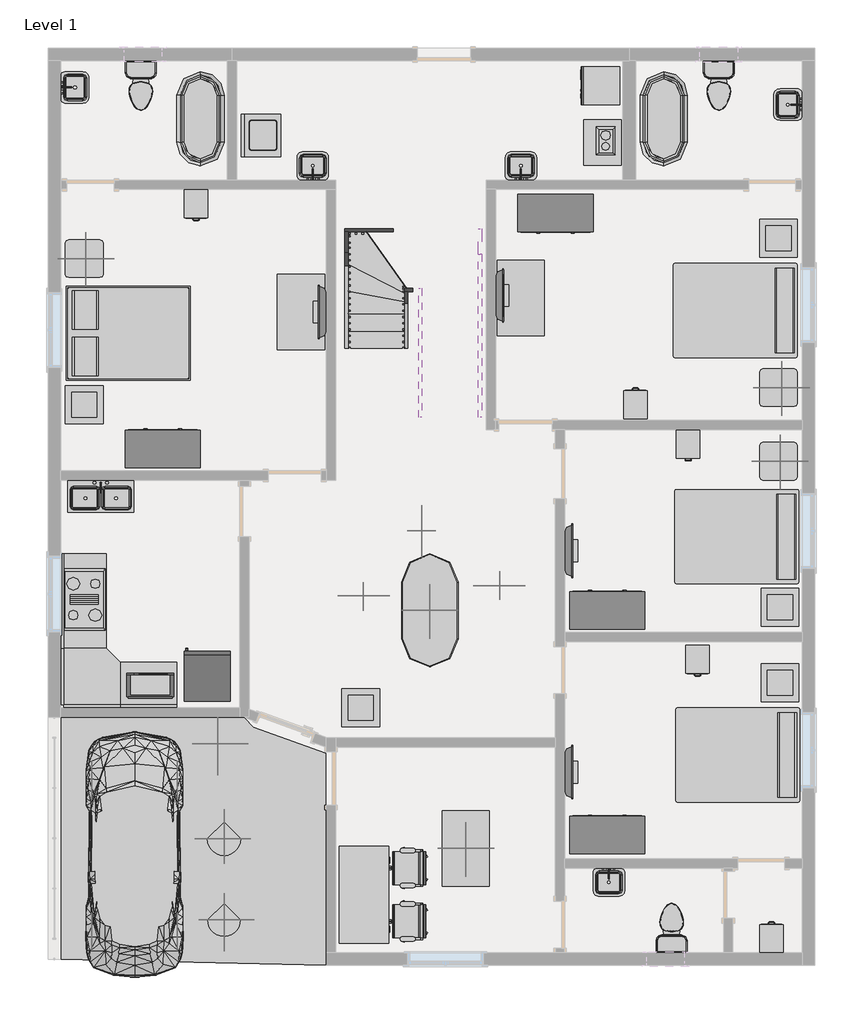
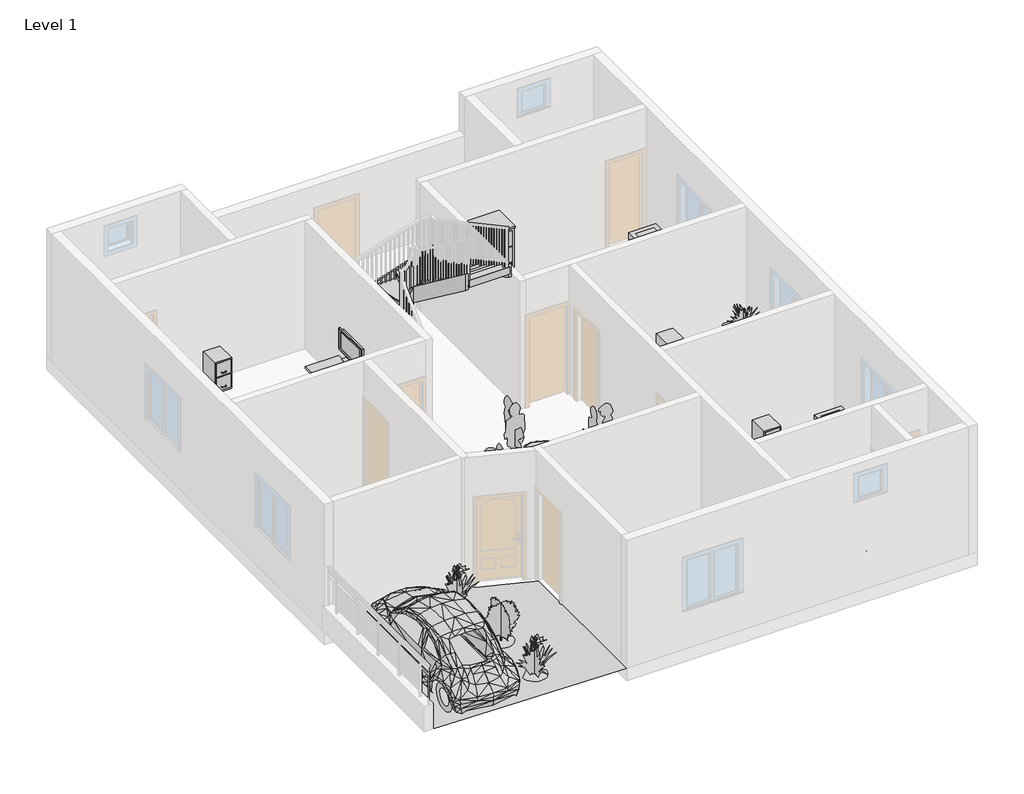
# One storey, part 3 of 3: 34 furniture elements, 15 flow terminals, 11 proxies, 8 geographic elements, 8 members, 1 stair flight.
"""IFC4 building model written with IfcOpenShell, lengths in millimetres."""

from ifc_helpers import new_model, si_unit, frame, origin, place, context, project, spatial, polyline, outline, extrude, triangles, transform, mapped, element, save
from components import proxy_fe84b772, proxy_bb1e6e30, proxy_45b28599, proxy_8a8d5ab2, rpc_beetle_rpc_beetle_3ce7ba48, rpc_female_69e001fa, proxy_a13a33b2, proxy_718fa39f, flow_terminal_2b63360b, flow_terminal_accce45a, flow_terminal_a53be723, flow_terminal_62a433f7, toilet_domestic_3d_toilet_domestic_3d_f7549cf7, toilet_domestic_3d_toilet_domestic_3d_183bbd19, flow_terminal_b374fae2, furniture_1d2926bd, furniture_e1791683, furniture_bb55ed6b, furniture_552c1472, chair_task_arms_chair_task_arms_fa5a08ef, furniture_072f6425, furniture_9fa109b2, furniture_56245f3a, furniture_b5c51a22, furniture_2c34a4f9, furniture_31d08a24, furniture_d260d85f, furniture_6a32cbcf, furniture_9653231d, rpc_plant_tropical_55f6ff97, rpc_plant_tropical_agave_1_5_93a2a214, rpc_plant_tropical_jungle_flame_3_9c4808c2, stair_flight_4b05d3ae

model = new_model("IFC4")

# Units and contexts
model_context = context("Model", 3, world=origin())
ifc_project = project(units=[si_unit("LENGTHUNIT", "METRE", prefix="MILLI")], contexts=[model_context])

# Site, building, storey
site = spatial("IfcSite", under=ifc_project)
building = spatial("IfcBuilding", under=site)
storey = spatial("IfcBuildingStorey", under=building, Name="Level 1", Elevation=0.0)

# Proxies
placement = place(None, origin())
element("IfcBuildingElementProxy", 1, Name="Building Element Proxy", at=placement, inside=storey, context=model_context, shape_type="Tessellation", body=[
    triangles([(-14773.0750122, 3106.6452576, 0.0), (-11814.7102386, 3106.6452576, 0.0), (-10480.4742371, 2547.8453545, 0.0), (-10480.4742371, 1684.245306, 0.0), (-10480.4742371, -906.5547667, 0.0), (-14773.0750122, -804.9547909, 0.0), (-10378.8746246, 1684.245306, 0.0), (-10378.8746246, 2547.8453545, 0.0), (-11521.9792694, 3081.190416, 0.0)], [[2, 4, 9], [4, 2, 6], [2, 1, 6], [4, 5, 7], [5, 4, 6], [3, 7, 8], [7, 3, 4], [3, 8, 9], [4, 3, 9]], closed=False),
])
proxy_shape = proxy_fe84b772(model_context)
element("IfcBuildingElementProxy", 2, Name="Cook Top-2 Unit : 12\" x 18\"", ObjectType="Cook Top-2 Unit : 12\" x 18\"", at=placement, inside=storey, context=model_context, shape_type="MappedRepresentation", body=[
    mapped(proxy_shape, transform((-6035.4744419, 12398.2204454, 0.0), x_axis=(1.0000000000000007, 0.0, 0.0), y_axis=(0.0, 1.0000000000000007, 0.0), z_axis=(0.0, 0.0, 1.0))),
])
proxy_2_shape = proxy_bb1e6e30(model_context)
element("IfcBuildingElementProxy", 3, Name="Cook Top-4 Unit : 36\" x 20\"", ObjectType="Cook Top-4 Unit : 36\" x 20\"", at=placement, inside=storey, context=model_context, shape_type="MappedRepresentation", body=[
    mapped(proxy_2_shape, transform((-14392.0744419, 5011.6452409, 0.0), x_axis=(0.0, 1.0, 0.0), y_axis=(-1.0, 0.0, 0.0), z_axis=(0.0, 0.0, 1.0))),
])
proxy_3_shape = proxy_45b28599(model_context)
element("IfcBuildingElementProxy", 4, Name="Dishwasher : 24\" x 24\" x 34\"", ObjectType="Dishwasher : 24\" x 24\" x 34\"", at=placement, inside=storey, context=model_context, shape_type="MappedRepresentation", body=[
    mapped(proxy_3_shape, transform((-6301.9240067, 13699.7627094, 0.0), x_axis=(0.0, -1.0000000000000004, 0.0), y_axis=(1.0000000000000004, 0.0, 0.0), z_axis=(0.0, 0.0, 1.0))),
])
proxy_4_shape = proxy_8a8d5ab2(model_context)
element("IfcBuildingElementProxy", 5, Name="Microwave : 30\" x 16\" x 18\"", ObjectType="Microwave : 30\" x 16\" x 18\"", at=placement, inside=storey, context=model_context, shape_type="MappedRepresentation", body=[
    mapped(proxy_4_shape, transform((-12824.9815646, 3261.5647351, 0.0), x_axis=(-1.0000000000000004, 0.0, 0.0), y_axis=(0.0, -1.0000000000000004, 0.0), z_axis=(0.0, 0.0, 1.0))),
])
rpc_beetle_rpc_beetle_shape = rpc_beetle_rpc_beetle_3ce7ba48(model_context)
element("IfcBuildingElementProxy", 6, Name="RPC Beetle : RPC Beetle", ObjectType="RPC Beetle : RPC Beetle", at=placement, inside=storey, context=model_context, shape_type="MappedRepresentation", body=[
    mapped(rpc_beetle_rpc_beetle_shape, transform((-13579.2744419, -347.7547591, 0.0), x_axis=(1.0, 0.0, 0.0), y_axis=(0.0, 1.0, 0.0), z_axis=(0.0, 0.0, 1.0))),
])
rpc_female_shape = rpc_female_69e001fa(model_context)
element("IfcBuildingElementProxy", 7, Name="RPC Female", ObjectType="RPC Female", at=placement, inside=storey, context=model_context, shape_type="MappedRepresentation", body=[
    mapped(rpc_female_shape, transform((-9721.6494419, 5062.4452409, 0.0), x_axis=(0.0, 1.0000000000000002, 0.0), y_axis=(-1.0000000000000002, 0.0, 0.0), z_axis=(0.0, 0.0, 1.0))),
])
element("IfcBuildingElementProxy", 8, Name="RPC Female", ObjectType="RPC Female", at=placement, inside=storey, context=model_context, shape_type="MappedRepresentation", body=[
    mapped(rpc_female_shape, transform((-8940.5994419, 5964.1452409, 0.0), x_axis=(1.0, 0.0, 0.0), y_axis=(0.0, 1.0, 0.0), z_axis=(0.0, 0.0, 1.0))),
])
element("IfcBuildingElementProxy", 9, Name="RPC Female", ObjectType="RPC Female", at=placement, inside=storey, context=model_context, shape_type="MappedRepresentation", body=[
    mapped(rpc_female_shape, transform((-7829.3494419, 5240.2452409, 0.0), x_axis=(0.0, -1.0000000000000007, 0.0), y_axis=(1.0000000000000007, 0.0, 0.0), z_axis=(0.0, 0.0, 1.0))),
])
proxy_5_shape = proxy_a13a33b2(model_context)
element("IfcBuildingElementProxy", 10, Name="Refrigerator : 30\" x 32\" RH", ObjectType="Refrigerator : 30\" x 32\" RH", at=placement, inside=storey, context=model_context, shape_type="MappedRepresentation", body=[
    mapped(proxy_5_shape, transform((-12402.9369419, 3753.1462695, 0.0), x_axis=(-1.0000000000000004, 0.0, 0.0), y_axis=(0.0, -1.0000000000000004, 0.0), z_axis=(0.0, 0.0, 1.0))),
])
proxy_6_shape = proxy_718fa39f(model_context)
element("IfcBuildingElementProxy", 11, Name="Washer : 27\" x 25\" x 35\"", ObjectType="Washer : 27\" x 25\" x 35\"", at=placement, inside=storey, context=model_context, shape_type="MappedRepresentation", body=[
    mapped(proxy_6_shape, transform((-11255.4248771, 12096.9277724, 0.0), x_axis=(0.0, 1.0000000000000004, 0.0), y_axis=(-1.0000000000000004, 0.0, 0.0), z_axis=(0.0, 0.0, 1.0))),
])

# Flow terminals
flow_terminal_shape = flow_terminal_2b63360b(model_context)
element("IfcFlowTerminal", 12, ObjectType="Floor Drain - Rectangular : 5\"x5\" Strainer - 2\" Drain", at=placement, inside=storey, context=model_context, shape_type="MappedRepresentation", body=[
    mapped(flow_terminal_shape, transform((-13122.0744419, 12022.0452409, 0.0), x_axis=(1.0, 0.0, 0.0), y_axis=(0.0, 1.0, 0.0), z_axis=(0.0, 0.0, 1.0))),
])
element("IfcFlowTerminal", 13, ObjectType="Floor Drain - Rectangular : 5\"x5\" Strainer - 2\" Drain", at=placement, inside=storey, context=model_context, shape_type="MappedRepresentation", body=[
    mapped(flow_terminal_shape, transform((-11598.0744419, 13368.2452409, 0.0), x_axis=(1.0, 0.0, 0.0), y_axis=(0.0, 1.0, 0.0), z_axis=(0.0, 0.0, 1.0))),
])
element("IfcFlowTerminal", 14, ObjectType="Floor Drain - Rectangular : 5\"x5\" Strainer - 2\" Drain", at=placement, inside=storey, context=model_context, shape_type="MappedRepresentation", body=[
    mapped(flow_terminal_shape, transform((-4460.6744419, 12225.2452409, 0.0), x_axis=(1.0, 0.0, 0.0), y_axis=(0.0, 1.0, 0.0), z_axis=(0.0, 0.0, 1.0))),
])
flow_terminal_2_shape = flow_terminal_accce45a(model_context)
element("IfcFlowTerminal", 15, ObjectType="Floor Drain - Round : 5\" Strainer - 2\" Drain", at=placement, inside=storey, context=model_context, shape_type="MappedRepresentation", body=[
    mapped(flow_terminal_2_shape, transform((-5425.8744419, -208.6587317, 0.0), x_axis=(1.0, 0.0, 0.0), y_axis=(0.0, 1.0, 0.0), z_axis=(0.0, 0.0, 1.0))),
])
flow_terminal_3_shape = flow_terminal_a53be723(model_context)
element("IfcFlowTerminal", 16, ObjectType="Sink Kitchen-Double : 42\" x 21\"", at=placement, inside=storey, context=model_context, shape_type="MappedRepresentation", body=[
    mapped(flow_terminal_3_shape, transform((-14141.0636825, 6685.6998398, 0.0), x_axis=(1.0, 0.0, 0.0), y_axis=(0.0, 1.0, 0.0), z_axis=(0.0, 0.0, 1.0))),
])
flow_terminal_4_shape = flow_terminal_62a433f7(model_context)
element("IfcFlowTerminal", 17, ObjectType="Sink Vanity-Square : 20\" x 18\"", at=placement, inside=storey, context=model_context, shape_type="MappedRepresentation", body=[
    mapped(flow_terminal_4_shape, transform((-14592.9290408, 13276.3560004, 0.0), x_axis=(0.0, 1.0000000000000002, 0.0), y_axis=(-1.0000000000000002, 0.0, 0.0), z_axis=(0.0, 0.0, 1.0))),
])
element("IfcFlowTerminal", 18, ObjectType="Sink Vanity-Square : 20\" x 18\"", at=placement, inside=storey, context=model_context, shape_type="MappedRepresentation", body=[
    mapped(flow_terminal_4_shape, transform((-10680.6852013, 11973.5906421, 0.0), x_axis=(-1.0, 0.0, 0.0), y_axis=(0.0, -1.0, 0.0), z_axis=(0.0, 0.0, 1.0))),
])
element("IfcFlowTerminal", 19, ObjectType="Sink Vanity-Square : 20\" x 18\"", at=placement, inside=storey, context=model_context, shape_type="MappedRepresentation", body=[
    mapped(flow_terminal_4_shape, transform((-7315.1852013, 11973.5906421, 0.0), x_axis=(-0.9999999999999998, 0.0, 0.0), y_axis=(0.0, -0.9999999999999998, 0.0), z_axis=(0.0, 0.0, 1.0))),
])
element("IfcFlowTerminal", 20, ObjectType="Sink Vanity-Square : 20\" x 18\"", at=placement, inside=storey, context=model_context, shape_type="MappedRepresentation", body=[
    mapped(flow_terminal_4_shape, transform((-2964.419843, 13028.3344815, 0.0), x_axis=(0.0, -1.0000000000000004, 0.0), y_axis=(1.0000000000000004, 0.0, 0.0), z_axis=(0.0, 0.0, 1.0))),
])
element("IfcFlowTerminal", 21, ObjectType="Sink Vanity-Square : 20\" x 18\"", at=placement, inside=storey, context=model_context, shape_type="MappedRepresentation", body=[
    mapped(flow_terminal_4_shape, transform((-5924.1636825, 488.0998398, 0.0), x_axis=(1.0, 0.0, 0.0), y_axis=(0.0, 1.0, 0.0), z_axis=(0.0, 0.0, 1.0))),
])
toilet_domestic_3d_toilet_domestic_3d_shape = toilet_domestic_3d_toilet_domestic_3d_f7549cf7(model_context)
toilet_domestic_3d_toilet_domestic_3d_2_shape = toilet_domestic_3d_toilet_domestic_3d_183bbd19(model_context)
element("IfcFlowTerminal", 22, ObjectType="Toilet-Domestic-3D : Toilet-Domestic-3D", at=placement, inside=storey, context=model_context, shape_type="MappedRepresentation", body=[
    mapped(toilet_domestic_3d_toilet_domestic_3d_shape, transform((-13477.6744419, 13229.1492136, 0.0), x_axis=(1.0, 0.0, 0.0), y_axis=(0.0, 1.0, 0.0), z_axis=(0.0, 0.0, 1.0))),
    mapped(toilet_domestic_3d_toilet_domestic_3d_2_shape, transform((-13477.6744419, 13229.1492136, 0.0), x_axis=(1.0, 0.0, 0.0), y_axis=(0.0, 1.0, 0.0), z_axis=(0.0, 0.0, 1.0))),
])
element("IfcFlowTerminal", 23, ObjectType="Toilet-Domestic-3D : Toilet-Domestic-3D", at=placement, inside=storey, context=model_context, shape_type="MappedRepresentation", body=[
    mapped(toilet_domestic_3d_toilet_domestic_3d_shape, transform((-4130.4744419, 13229.1492136, 0.0), x_axis=(1.0, 0.0, 0.0), y_axis=(0.0, 1.0, 0.0), z_axis=(0.0, 0.0, 1.0))),
    mapped(toilet_domestic_3d_toilet_domestic_3d_2_shape, transform((-4130.4744419, 13229.1492136, 0.0), x_axis=(1.0, 0.0, 0.0), y_axis=(0.0, 1.0, 0.0), z_axis=(0.0, 0.0, 1.0))),
])
element("IfcFlowTerminal", 24, ObjectType="Toilet-Domestic-3D : Toilet-Domestic-3D", at=placement, inside=storey, context=model_context, shape_type="MappedRepresentation", body=[
    mapped(toilet_domestic_3d_toilet_domestic_3d_shape, transform((-4892.4744419, -208.6587317, 0.0), x_axis=(-1.0000000000000004, 0.0, 0.0), y_axis=(0.0, -1.0000000000000004, 0.0), z_axis=(0.0, 0.0, 1.0))),
    mapped(toilet_domestic_3d_toilet_domestic_3d_2_shape, transform((-4892.4744419, -208.6587317, 0.0), x_axis=(-1.0000000000000004, 0.0, 0.0), y_axis=(0.0, -1.0000000000000004, 0.0), z_axis=(0.0, 0.0, 1.0))),
])
flow_terminal_5_shape = flow_terminal_b374fae2(model_context)
element("IfcFlowTerminal", 25, ObjectType="Tub-Free Standing-3D : 30\" x 60\"", at=placement, inside=storey, context=model_context, shape_type="MappedRepresentation", body=[
    mapped(flow_terminal_5_shape, transform((-12512.4744419, 12784.0452409, 0.0), x_axis=(1.0, 0.0, 0.0), y_axis=(0.0, 1.0, 0.0), z_axis=(0.0, 0.0, 1.0))),
])
element("IfcFlowTerminal", 26, ObjectType="Tub-Free Standing-3D : 30\" x 60\"", at=placement, inside=storey, context=model_context, shape_type="MappedRepresentation", body=[
    mapped(flow_terminal_5_shape, transform((-5019.4744419, 12784.0452409, 0.0), x_axis=(1.0, 0.0, 0.0), y_axis=(0.0, 1.0, 0.0), z_axis=(0.0, 0.0, 1.0))),
])

# Furniture
furniture_shape = furniture_1d2926bd(model_context)
element("IfcFurniture", 27, ObjectType="Bed-Box : Queen 60\" x 79\"", at=placement, inside=storey, context=model_context, shape_type="MappedRepresentation", body=[
    mapped(furniture_shape, transform((-13915.3039501, 8977.7927819, 0.0), x_axis=(0.0, 1.0000000000000002, 0.0), y_axis=(-1.0000000000000002, 0.0, 0.0), z_axis=(0.0, 0.0, 1.0))),
])
furniture_2_shape = furniture_e1791683(model_context)
element("IfcFurniture", 28, ObjectType="Bed-Standard.0001 : Queen 60\" x 79\"", at=placement, inside=storey, context=model_context, shape_type="MappedRepresentation", body=[
    mapped(furniture_2_shape, transform((-3818.1793599, 9956.7337655, 0.0), x_axis=(0.0, -1.0, 0.0), y_axis=(1.0, 0.0, 0.0), z_axis=(0.0, 0.0, 1.0))),
])
element("IfcFurniture", 29, ObjectType="Bed-Standard.0001 : Queen 60\" x 79\"", at=placement, inside=storey, context=model_context, shape_type="MappedRepresentation", body=[
    mapped(furniture_2_shape, transform((-3792.7793599, 6299.1337655, 0.0), x_axis=(0.0, -1.0000000000000002, 0.0), y_axis=(1.0000000000000002, 0.0, 0.0), z_axis=(0.0, 0.0, 1.0))),
])
element("IfcFurniture", 30, ObjectType="Bed-Standard.0001 : Queen 60\" x 79\"", at=placement, inside=storey, context=model_context, shape_type="MappedRepresentation", body=[
    mapped(furniture_2_shape, transform((-3780.0793599, 2768.5337655, 0.0), x_axis=(0.0, -1.0, 0.0), y_axis=(1.0, 0.0, 0.0), z_axis=(0.0, 0.0, 1.0))),
])
furniture_3_shape = furniture_bb55ed6b(model_context)
element("IfcFurniture", 31, ObjectType="Cabinet-File 2 Drawer : 15\" x 18\"", at=placement, inside=storey, context=model_context, shape_type="MappedRepresentation", body=[
    mapped(furniture_3_shape, transform((-12454.7220198, 11554.5795411, 0.0), x_axis=(1.0, 0.0, 0.0), y_axis=(0.0, 1.0, 0.0), z_axis=(0.0, 0.0, 1.0))),
])
element("IfcFurniture", 32, ObjectType="Cabinet-File 2 Drawer : 15\" x 18\"", at=placement, inside=storey, context=model_context, shape_type="MappedRepresentation", body=[
    mapped(furniture_3_shape, transform((-5604.5708889, 8019.1109408, 0.0), x_axis=(-1.0, 0.0, 0.0), y_axis=(0.0, -1.0, 0.0), z_axis=(0.0, 0.0, 1.0))),
])
element("IfcFurniture", 33, ObjectType="Cabinet-File 2 Drawer : 15\" x 18\"", at=placement, inside=storey, context=model_context, shape_type="MappedRepresentation", body=[
    mapped(furniture_3_shape, transform((-4497.8779949, 7668.3795411, 0.0), x_axis=(1.0, 0.0, 0.0), y_axis=(0.0, 1.0, 0.0), z_axis=(0.0, 0.0, 1.0))),
])
element("IfcFurniture", 34, ObjectType="Cabinet-File 2 Drawer : 15\" x 18\"", at=placement, inside=storey, context=model_context, shape_type="MappedRepresentation", body=[
    mapped(furniture_3_shape, transform((-4345.4779949, 4188.5795411, 0.0), x_axis=(1.0, 0.0, 0.0), y_axis=(0.0, 1.0, 0.0), z_axis=(0.0, 0.0, 1.0))),
])
furniture_4_shape = furniture_552c1472(model_context)
element("IfcFurniture", 35, ObjectType="Cabinet-File 3 Drawer : 15\" x 18\"", at=placement, inside=storey, context=model_context, shape_type="MappedRepresentation", body=[
    mapped(furniture_4_shape, transform((-3407.4708889, -616.8890592, 0.0), x_axis=(-1.0000000000000004, 0.0, 0.0), y_axis=(0.0, -1.0000000000000004, 0.0), z_axis=(0.0, 0.0, 1.0))),
])
chair_task_arms_chair_task_arms_shape = chair_task_arms_chair_task_arms_fa5a08ef(model_context)
element("IfcFurniture", 36, ObjectType="Chair-Task Arms : Chair-Task Arms", at=placement, inside=storey, context=model_context, shape_type="MappedRepresentation", body=[
    mapped(chair_task_arms_chair_task_arms_shape, transform((-9115.3285403, -336.3455787, 0.0), x_axis=(0.0, 1.0, 0.0), y_axis=(-1.0, 0.0, 0.0), z_axis=(0.0, 0.0, 1.0))),
])
element("IfcFurniture", 37, ObjectType="Chair-Task Arms : Chair-Task Arms", at=placement, inside=storey, context=model_context, shape_type="MappedRepresentation", body=[
    mapped(chair_task_arms_chair_task_arms_shape, transform((-9115.3285403, 527.2544213, 0.0), x_axis=(0.0, 1.0000000000000002, 0.0), y_axis=(-1.0000000000000002, 0.0, 0.0), z_axis=(0.0, 0.0, 1.0))),
])
furniture_5_shape = furniture_072f6425(model_context)
element("IfcFurniture", 38, ObjectType="Desk : 60\" x 30\" Student", at=placement, inside=storey, context=model_context, shape_type="MappedRepresentation", body=[
    mapped(furniture_5_shape, transform((-10251.8744419, 998.4452409, 0.0), x_axis=(0.0, -1.0000000000000007, 0.0), y_axis=(1.0000000000000007, 0.0, 0.0), z_axis=(0.0, 0.0, 1.0))),
])
furniture_6_shape = furniture_9fa109b2(model_context)
element("IfcFurniture", 39, ObjectType="Dresser : 48\" x 72\" x 24\"", at=placement, inside=storey, context=model_context, shape_type="MappedRepresentation", body=[
    mapped(furniture_6_shape, transform((-13391.2677017, 7083.150595, 0.0), x_axis=(-1.0000000000000004, 0.0, 0.0), y_axis=(0.0, -1.0000000000000004, 0.0), z_axis=(0.0, 0.0, 1.0))),
])
element("IfcFurniture", 40, ObjectType="Dresser : 48\" x 72\" x 24\"", at=placement, inside=storey, context=model_context, shape_type="MappedRepresentation", body=[
    mapped(furniture_6_shape, transform((-6502.8811821, 11623.208195, 0.0), x_axis=(1.0, 0.0, 0.0), y_axis=(0.0, 1.0, 0.0), z_axis=(0.0, 0.0, 1.0))),
])
element("IfcFurniture", 41, ObjectType="Dresser : 48\" x 72\" x 24\"", at=placement, inside=storey, context=model_context, shape_type="MappedRepresentation", body=[
    mapped(furniture_6_shape, transform((-6203.0677017, 4470.6822868, 0.0), x_axis=(-1.0000000000000004, 0.0, 0.0), y_axis=(0.0, -1.0000000000000004, 0.0), z_axis=(0.0, 0.0, 1.0))),
])
element("IfcFurniture", 42, ObjectType="Dresser : 48\" x 72\" x 24\"", at=placement, inside=storey, context=model_context, shape_type="MappedRepresentation", body=[
    mapped(furniture_6_shape, transform((-6203.0677017, 838.4822868, 0.0), x_axis=(-1.0000000000000004, 0.0, 0.0), y_axis=(0.0, -1.0000000000000004, 0.0), z_axis=(0.0, 0.0, 1.0))),
])
furniture_7_shape = furniture_56245f3a(model_context)
element("IfcFurniture", 43, ObjectType="TV - Flat Screen : 32\"", at=placement, inside=storey, context=model_context, shape_type="MappedRepresentation", body=[
    mapped(furniture_7_shape, transform((-10539.0130656, 9655.9007268, 914.4), x_axis=(0.0, -1.0000000000000004, 0.0), y_axis=(1.0000000000000004, 0.0, 0.0), z_axis=(0.0, 0.0, 1.0))),
])
element("IfcFurniture", 44, ObjectType="TV - Flat Screen : 32\"", at=placement, inside=storey, context=model_context, shape_type="MappedRepresentation", body=[
    mapped(furniture_7_shape, transform((-7678.7358183, 9930.4897551, 990.6), x_axis=(0.0, 1.0000000000000002, 0.0), y_axis=(-1.0000000000000002, 0.0, 0.0), z_axis=(0.0, 0.0, 1.0))),
])
element("IfcFurniture", 45, ObjectType="TV - Flat Screen : 32\"", at=placement, inside=storey, context=model_context, shape_type="MappedRepresentation", body=[
    mapped(furniture_7_shape, transform((-6561.1358183, 5802.9897551, 914.4), x_axis=(0.0, 1.0, 0.0), y_axis=(-1.0, 0.0, 0.0), z_axis=(0.0, 0.0, 1.0))),
])
element("IfcFurniture", 46, ObjectType="TV - Flat Screen : 32\"", at=placement, inside=storey, context=model_context, shape_type="MappedRepresentation", body=[
    mapped(furniture_7_shape, transform((-6561.1358183, 2221.5897551, 914.4), x_axis=(0.0, 1.0, 0.0), y_axis=(-1.0, 0.0, 0.0), z_axis=(0.0, 0.0, 1.0))),
])
furniture_8_shape = furniture_b5c51a22(model_context)
element("IfcFurniture", 47, ObjectType="Table-Coffee : 24\" x 24\" x 24\"", at=placement, inside=storey, context=model_context, shape_type="MappedRepresentation", body=[
    mapped(furniture_8_shape, transform((-14410.3402086, 8066.0341631, 0.0), x_axis=(1.0, 0.0, 0.0), y_axis=(0.0, 1.0, 0.0), z_axis=(0.0, 0.0, 1.0))),
])
element("IfcFurniture", 48, ObjectType="Table-Coffee : 24\" x 24\" x 24\"", at=placement, inside=storey, context=model_context, shape_type="MappedRepresentation", body=[
    mapped(furniture_8_shape, transform((-3183.5402086, 10758.4341631, 0.0), x_axis=(1.0, 0.0, 0.0), y_axis=(0.0, 1.0, 0.0), z_axis=(0.0, 0.0, 1.0))),
])
element("IfcFurniture", 49, ObjectType="Table-Coffee : 24\" x 24\" x 24\"", at=placement, inside=storey, context=model_context, shape_type="MappedRepresentation", body=[
    mapped(furniture_8_shape, transform((-9939.9402086, 3163.8341631, 0.0), x_axis=(1.0, 0.0, 0.0), y_axis=(0.0, 1.0, 0.0), z_axis=(0.0, 0.0, 1.0))),
])
element("IfcFurniture", 50, ObjectType="Table-Coffee : 24\" x 24\" x 24\"", at=placement, inside=storey, context=model_context, shape_type="MappedRepresentation", body=[
    mapped(furniture_8_shape, transform((-3158.1402086, 4789.4341631, 0.0), x_axis=(1.0, 0.0, 0.0), y_axis=(0.0, 1.0, 0.0), z_axis=(0.0, 0.0, 1.0))),
])
element("IfcFurniture", 51, ObjectType="Table-Coffee : 24\" x 24\" x 24\"", at=placement, inside=storey, context=model_context, shape_type="MappedRepresentation", body=[
    mapped(furniture_8_shape, transform((-3158.1402086, 3570.2341631, 0.0), x_axis=(1.0, 0.0, 0.0), y_axis=(0.0, 1.0, 0.0), z_axis=(0.0, 0.0, 1.0))),
])
furniture_9_shape = furniture_2c34a4f9(model_context)
element("IfcFurniture", 52, ObjectType="Table-Dining Oval : 36\" x 72\"", at=placement, inside=storey, context=model_context, shape_type="MappedRepresentation", body=[
    mapped(furniture_9_shape, transform((-9162.1728026, 5235.6649131, 0.0), x_axis=(0.0, 1.0, 0.0), y_axis=(-1.0, 0.0, 0.0), z_axis=(0.0, 0.0, 1.0))),
])
furniture_10_shape = furniture_31d08a24(model_context)
element("IfcFurniture", 53, ObjectType="Table-End : 24\" x 24\"", at=placement, inside=storey, context=model_context, shape_type="MappedRepresentation", body=[
    mapped(furniture_10_shape, transform((-14700.6080722, 10371.0452409, 0.0), x_axis=(1.0, 0.0, 0.0), y_axis=(0.0, 1.0, 0.0), z_axis=(0.0, 0.0, 1.0))),
])
element("IfcFurniture", 54, ObjectType="Table-End : 24\" x 24\"", at=placement, inside=storey, context=model_context, shape_type="MappedRepresentation", body=[
    mapped(furniture_10_shape, transform((-3473.8080722, 8284.5135491, 0.0), x_axis=(1.0, 0.0, 0.0), y_axis=(0.0, 1.0, 0.0), z_axis=(0.0, 0.0, 1.0))),
])
element("IfcFurniture", 55, ObjectType="Table-End : 24\" x 24\"", at=placement, inside=storey, context=model_context, shape_type="MappedRepresentation", body=[
    mapped(furniture_10_shape, transform((-3473.8080722, 7094.4452409, 0.0), x_axis=(1.0, 0.0, 0.0), y_axis=(0.0, 1.0, 0.0), z_axis=(0.0, 0.0, 1.0))),
])
furniture_11_shape = furniture_d260d85f(model_context)
element("IfcFurniture", 56, ObjectType="Table-Rectangular : 72\" x 30\" 2", at=placement, inside=storey, context=model_context, shape_type="MappedRepresentation", body=[
    mapped(furniture_11_shape, transform((-10886.8744419, 9659.8452409, 0.0), x_axis=(0.0, 1.0000000000000002, 0.0), y_axis=(-1.0000000000000002, 0.0, 0.0), z_axis=(0.0, 0.0, 1.0))),
])
element("IfcFurniture", 57, ObjectType="Table-Rectangular : 72\" x 30\" 2", at=placement, inside=storey, context=model_context, shape_type="MappedRepresentation", body=[
    mapped(furniture_11_shape, transform((-7330.8744419, 9888.4452409, 0.0), x_axis=(0.0, 1.0000000000000002, 0.0), y_axis=(-1.0000000000000002, 0.0, 0.0), z_axis=(0.0, 0.0, 1.0))),
])
element("IfcFurniture", 58, ObjectType="Table-Rectangular : 72\" x 30\" 2", at=placement, inside=storey, context=model_context, shape_type="MappedRepresentation", body=[
    mapped(furniture_11_shape, transform((-8219.8744419, 985.7452409, 0.0), x_axis=(0.0, 1.0, 0.0), y_axis=(-1.0, 0.0, 0.0), z_axis=(0.0, 0.0, 1.0))),
])
furniture_12_shape = furniture_6a32cbcf(model_context)
element("IfcFurniture", 59, ObjectType="Table-Rectangular : 72\" x 30\" 3", at=placement, inside=storey, context=model_context, shape_type="MappedRepresentation", body=[
    mapped(furniture_12_shape, transform((-6010.0744419, 12403.0452409, 0.0), x_axis=(0.0, 1.0, 0.0), y_axis=(-1.0, 0.0, 0.0), z_axis=(0.0, 0.0, 1.0))),
])
furniture_13_shape = furniture_9653231d(model_context)
element("IfcFurniture", 60, ObjectType="Work Station Cubicle : 96\" x 96\"", at=placement, inside=storey, context=model_context, shape_type="MappedRepresentation", body=[
    mapped(furniture_13_shape, transform((-15268.0974495, 3390.7769932, 0.0), x_axis=(0.0, 1.0000000000000002, 0.0), y_axis=(-1.0000000000000002, 0.0, 0.0), z_axis=(0.0, 0.0, 1.0))),
])

# Geographic elements
rpc_plant_tropical_shape = rpc_plant_tropical_55f6ff97(model_context)
element("IfcGeographicElement", 61, ObjectType="RPC Plant - Tropical", at=placement, inside=storey, context=model_context, shape_type="MappedRepresentation", body=[
    mapped(rpc_plant_tropical_shape, transform((-12233.0744419, 2674.8452409, 0.0), x_axis=(1.0, 0.0, 0.0), y_axis=(0.0, 1.0, 0.0), z_axis=(0.0, 0.0, 1.0))),
])
element("IfcGeographicElement", 62, ObjectType="RPC Plant - Tropical", at=placement, inside=storey, context=model_context, shape_type="MappedRepresentation", body=[
    mapped(rpc_plant_tropical_shape, transform((-12131.4744419, -169.9547591, 0.0), x_axis=(1.0, 0.0, 0.0), y_axis=(0.0, 1.0, 0.0), z_axis=(0.0, 0.0, 1.0))),
])
rpc_plant_tropical_agave_1_5_shape = rpc_plant_tropical_agave_1_5_93a2a214(model_context)
element("IfcGeographicElement", 63, ObjectType="RPC Plant - Tropical : Agave - 1.5'", at=placement, inside=storey, context=model_context, shape_type="MappedRepresentation", body=[
    mapped(rpc_plant_tropical_agave_1_5_shape, transform((-14366.6744419, 10523.4452409, 609.6), x_axis=(1.0, 0.0, 0.0), y_axis=(0.0, 1.0, 0.0), z_axis=(0.0, 0.0, 1.0))),
])
element("IfcGeographicElement", 64, ObjectType="RPC Plant - Tropical : Agave - 1.5'", at=placement, inside=storey, context=model_context, shape_type="MappedRepresentation", body=[
    mapped(rpc_plant_tropical_agave_1_5_shape, transform((-3114.4744419, 8436.9135491, 609.6), x_axis=(1.0, 0.0, 0.0), y_axis=(0.0, 1.0, 0.0), z_axis=(0.0, 0.0, 1.0))),
])
element("IfcGeographicElement", 65, ObjectType="RPC Plant - Tropical : Agave - 1.5'", at=placement, inside=storey, context=model_context, shape_type="MappedRepresentation", body=[
    mapped(rpc_plant_tropical_agave_1_5_shape, transform((-8804.0744419, 4833.8452409, 609.6), x_axis=(1.0, 0.0, 0.0), y_axis=(0.0, 1.0, 0.0), z_axis=(0.0, 0.0, 1.0))),
])
element("IfcGeographicElement", 66, ObjectType="RPC Plant - Tropical : Agave - 1.5'", at=placement, inside=storey, context=model_context, shape_type="MappedRepresentation", body=[
    mapped(rpc_plant_tropical_agave_1_5_shape, transform((-3139.8744419, 7246.8452409, 609.6), x_axis=(1.0, 0.0, 0.0), y_axis=(0.0, 1.0, 0.0), z_axis=(0.0, 0.0, 1.0))),
])
element("IfcGeographicElement", 67, ObjectType="RPC Plant - Tropical : Agave - 1.5'", at=placement, inside=storey, context=model_context, shape_type="MappedRepresentation", body=[
    mapped(rpc_plant_tropical_agave_1_5_shape, transform((-8219.8744419, 985.7452409, 685.8), x_axis=(1.0, 0.0, 0.0), y_axis=(0.0, 1.0, 0.0), z_axis=(0.0, 0.0, 1.0))),
])
rpc_plant_tropical_jungle_flame_3_shape = rpc_plant_tropical_jungle_flame_3_9c4808c2(model_context)
element("IfcGeographicElement", 68, ObjectType="RPC Plant - Tropical : Jungle Flame - 3'", at=placement, inside=storey, context=model_context, shape_type="MappedRepresentation", body=[
    mapped(rpc_plant_tropical_jungle_flame_3_shape, transform((-12131.4744419, 1138.1452409, 0.0), x_axis=(1.0, 0.0, 0.0), y_axis=(0.0, 1.0, 0.0), z_axis=(0.0, 0.0, 1.0))),
])

# Members
element("IfcMember", 69, ObjectType="Stringer - 2\" Width", at=placement, inside=storey, context=model_context, shape_type="SweptSolid", body=[
    extrude(outline(polyline([(9071.9135491, 241.2701641), (9071.9135491, 577.8751786), (10617.0071098, 1301.9005649), (10617.0071098, 965.2955504), (9071.9135491, 241.2701641)])), frame((-10175.6744419, 0.0, 0.0), z_axis=(1.0, 0.0, 0.0), x_axis=(0.0, 1.0, 0.0)), (0.0, 0.0, 1.0), 50.8),
])
element("IfcMember", 70, ObjectType="Stringer - 2\" Width", at=placement, inside=storey, context=model_context, shape_type="SweptSolid", body=[
    extrude(outline(polyline([(-10124.8744419, 10617.0071098), (-10175.6744419, 10617.0071098), (-10175.6744419, 10955.2452409), (-10124.8744419, 10955.2452409), (-10124.8744419, 10617.0071098)])), frame((0.0, 0.0, 965.2955504), z_axis=(0.0, 0.0, 1.0), x_axis=(1.0, 0.0, 0.0)), (0.0, 0.0, 1.0), 336.6050145),
])
element("IfcMember", 71, ObjectType="Stringer - 2\" Width", at=placement, inside=storey, context=model_context, shape_type="SweptSolid", body=[
    extrude(outline(polyline([(1285.6001408, -10175.6744419), (997.1005649, -10175.6744419), (997.1005649, -10025.7546446), (1641.7631511, -8016.6744419), (1969.9972697, -8016.6744419), (1969.9972697, -8042.7621994), (1285.6001408, -10175.6744419)])), frame((0.0, 10955.2452409, 0.0), z_axis=(0.0, 1.0, 0.0), x_axis=(0.0, 0.0, 1.0)), (0.0, 0.0, 1.0), 50.8),
])
element("IfcMember", 72, ObjectType="Stringer - 2\" Width", at=placement, inside=storey, context=model_context, shape_type="SweptSolid", body=[
    extrude(outline(polyline([(-8016.6744419, 11006.0452409), (-7965.8744419, 11006.0452409), (-7965.8744419, 10593.4694397), (-8016.6744419, 10593.4694397), (-8016.6744419, 11006.0452409)])), frame((0.0, 0.0, 1649.8904473), z_axis=(0.0, 0.0, 1.0), x_axis=(1.0, 0.0, 0.0)), (0.0, 0.0, 1.0), 320.1068224),
])
element("IfcMember", 73, ObjectType="Stringer - 2\" Width", at=placement, inside=storey, context=model_context, shape_type="SweptSolid", body=[
    extrude(outline(polyline([(10593.4694397, 1969.9972697), (10593.4694397, 1649.8904473), (7954.3135491, 3070.7452044), (7954.3135491, 3390.8520268), (10593.4694397, 1969.9972697)])), frame((-8016.6744419, 0.0, 0.0), z_axis=(1.0, 0.0, 0.0), x_axis=(0.0, 1.0, 0.0)), (0.0, 0.0, 1.0), 50.8),
])
element("IfcMember", 74, ObjectType="Stringer - 2\" Width", at=placement, inside=storey, context=model_context, shape_type="SweptSolid", body=[
    extrude(outline(polyline([(9071.9135491, 61.3897561), (9071.9135491, 489.3391875), (9990.0452409, 1394.2045547), (9990.0452409, 966.2551233), (9071.9135491, 61.3897561)])), frame((-9210.4744419, 0.0, 0.0), z_axis=(1.0, 0.0, 0.0), x_axis=(0.0, 1.0, 0.0)), (0.0, 0.0, 1.0), 50.8),
])
element("IfcMember", 75, ObjectType="Stringer - 2\" Width", at=placement, inside=storey, context=model_context, shape_type="SweptSolid", body=[
    extrude(outline(polyline([(1573.2682978, -9210.4744419), (1016.3211008, -9210.4744419), (1016.3211008, -9183.4001798), (1360.465107, -8981.8744419), (1918.7074486, -8981.8744419), (1918.7074486, -9008.1902861), (1573.2682978, -9210.4744419)])), frame((0.0, 9990.0452409, 0.0), z_axis=(0.0, 1.0, 0.0), x_axis=(0.0, 0.0, 1.0)), (0.0, 0.0, 1.0), 50.8),
])
element("IfcMember", 76, ObjectType="Stringer - 2\" Width", at=placement, inside=storey, context=model_context, shape_type="SweptSolid", body=[
    extrude(outline(polyline([(10040.8452409, 1918.7074486), (10040.8452409, 1537.60419), (7954.3135491, 3103.6807835), (7954.3135491, 3484.7840422), (10040.8452409, 1918.7074486)])), frame((-8981.8744419, 0.0, 0.0), z_axis=(1.0, 0.0, 0.0), x_axis=(0.0, 1.0, 0.0)), (0.0, 0.0, 1.0), 50.8),
])

# Stair flight
stair_flight_shape = stair_flight_4b05d3ae(model_context)
element("IfcStairFlight", 77, ObjectType="2\" Tread 1\" Nosing 1/4\" Riser", at=placement, inside=storey, context=model_context, shape_type="MappedRepresentation", body=[
    mapped(stair_flight_shape, transform((0.0, 0.0, 0.0), x_axis=(1.0, 0.0, 0.0), y_axis=(0.0, 1.0, 0.0), z_axis=(0.0, 0.0, 1.0))),
])

save(model, "model.ifc")

# Revit data of these elements
# Type "Cook Top-2 Unit : 12\" x 18\""
#   Assembly Code = "E1090400"
#   Counter Height = 3' - 0"
#   Depth = 1' - 6"
#   Width = 1' - 0"
#   Burner Material = Steel, Chrome Plated
#   Cooktop Material = Steel, Polished
#   Default Elevation = 0
# Type "Cook Top-4 Unit : 36\" x 20\""
#   Assembly Code = "E1090400"
#   Depth = 2' - 0"
#   Width = 3' - 0"
#   Burner Material = Steel, Chrome Plated
#   Cooktop Material = Steel, Polished
#   Default Elevation = 0
# Type "Dishwasher : 24\" x 24\" x 34\""
#   Label = "DW"
#   Assembly Code = "E1090400"
#   Depth = 2' - 0"
#   Height = 2' - 10"
#   Width = 2' - 0"
#   Dishwasher Material = Steel, Paint Finish, Ivory, Glossy
#   Panel Face Material = Plastic, Opaque Black
#   Default Elevation = 0
# Type "Microwave : 30\" x 16\" x 18\""
#   Assembly Code = "E1090400"
#   Depth = 1' - 4"
#   Height = 1' - 6"
#   Width = 2' - 6"
#   Microwave Material = Laminate, Ivory, Matte
#   Default Elevation = 0
# Type "RPC Beetle : RPC Beetle"
#   built-in parameter 1005195 = "RPC-16-0U6E-L4EG-ENH1-J3KF-SVEL-0TX4-C0"
#   Height = 0
# Type "RPC Female"
#   built-in parameter 1005195 = "RPC-8-FXA2-QQQ0-UGV2-6"
#   Height = 0
# Type "Refrigerator : 30\" x 32\" RH"
#   Label = "REF."
#   Assembly Code = "E1090400"
#   Depth = 2' - 7 3/4"
#   Handle = 2' - 3"
#   Height = 5' - 10"
#   Rear Clearance = 0' - 2"
#   Top Door Height = 1' - 8"
#   Width = 2' - 5 3/8"
#   Material = Steel, Paint Finish, Ivory, Glossy
#   Default Elevation = 0
# Type "Washer : 27\" x 25\" x 35\""
#   Label = "W"
#   Assembly Code = "E1090400"
#   Depth = 2' - 1"
#   Height = 2' - 11"
#   Width = 2' - 3"
#   Washer Material = Steel, Paint Finish, Ivory, Matte
#   Default Elevation = 0
# Type "Floor Drain - Rectangular : 5\"x5\" Strainer - 2\" Drain"
#   WFU = 2
#   Strainer Height = 0' - 3 1/4"
#   Half Strainer Length = 0' - 2 1/2"
#   Strainer Length = 0' - 5"
#   Radius 2 = 0' - 3.04167"
#   Radius 1 = 0' - 2.02083"
#   Radius 3 = 0' - 2 1/32"
#   Pipe Radius = 1"
#   Pipe Diameter = 2"
#   Height 2 = 0' - 0.725"
#   Height 1 = 0' - 1 13/16"
#   Body Radius = 0' - 4 1/16"
#   Body Height = 0' - 3 5/8"
#   Body Diameter = 0' - 8 1/8"
#   Drain Material = none
#   HWFU = 0
#   Default Elevation = 0
#   CWFU = 0
# Type "Floor Drain - Round : 5\" Strainer - 2\" Drain"
#   WFU = 2
#   Strainer Height = 0' - 3 1/4"
#   Strainer Radius = 0' - 2 1/2"
#   Strainer Diameter = 0' - 5"
#   Radius 6 = 0' - 0 5/8"
#   Radius 5 = 0' - 1 1/4"
#   Radius 4 = 0' - 1 7/8"
#   Radius 2 = 0' - 3.04167"
#   Radius 1 = 0' - 2.02083"
#   Radius 3 = 0' - 2 1/32"
#   Pipe Radius = 1"
#   Pipe Diameter = 2"
#   Height 2 = 0' - 0.725"
#   Height 1 = 0' - 1 13/16"
#   Body Radius = 0' - 4 1/16"
#   Body Height = 0' - 3 5/8"
#   Body Diameter = 0' - 8 1/8"
#   Drain Material = none
#   HWFU = 0
#   Default Elevation = 0
#   CWFU = 0
# Type "Sink Kitchen-Double : 42\" x 21\""
#   Assembly Code = "D2010410"
#   Counter Height = 3' - 0"
#   Depth = 1' - 9"
#   Width = 3' - 6"
#   Faucet Material = Steel, Polished
#   Sink Material = Steel, Polished
#   Default Elevation = 0
# Type "Sink Vanity-Square : 20\" x 18\""
#   Assembly Code = "D2010400"
#   Counter Height = 2' - 7"
#   Depth = 1' - 6"
#   Width = 1' - 8"
#   Basin Material = Porcelain, Linen
#   Faucet Material = Steel, Polished
#   Default Elevation = 0
# Type "Toilet-Domestic-3D : Toilet-Domestic-3D"
#   Assembly Code = "D2010110"
#   Toilet - Bowl/Basin Material = Porcelain, Linen
#   Toilet - Seat Material = Laminate, Linen, Matte
#   Default Elevation = 0
# Type "Tub-Free Standing-3D : 30\" x 60\""
#   Assembly Code = "D2010110"
#   Height = 1' - 6"
#   Length = 5' - 0"
#   Width = 2' - 6"
#   Tub Material = Porcelain, Ivory
#   Default Elevation = 0
# Type "Bed-Box : Queen 60\" x 79\""
#   Assembly Code = "E2020200"
#   Length = 6' - 7"
#   Width = 5' - 0"
#   Frame Material = Birch
#   Mattress Material = Linen, White
#   Default Elevation = 0
# Type "Bed-Standard.0001 : Queen 60\" x 79\""
#   Assembly Code = "E2020200"
#   Length = 6' - 7"
#   Width = 5' - 0"
#   Leg Material = Steel, Chrome Plated
#   Mattress Material = Linen, White
#   Default Elevation = 0
# Type "Cabinet-File 2 Drawer : 15\" x 18\""
#   Assembly Code = "E2020200"
#   Depth = 1' - 6"
#   Height = 2' - 5"
#   Width = 1' - 3"
#   Cabinet Material = Steel, Paint Finish, Ivory, Glossy
#   Handle Material = Steel, Chrome Plated
#   Default Elevation = 0
# Type "Cabinet-File 3 Drawer : 15\" x 18\""
#   Assembly Code = "E2020200"
#   Depth = 1' - 6"
#   Height = 3' - 5"
#   Width = 1' - 3"
#   Cabinet Material = Steel, Paint Finish, Ivory, Glossy
#   Handle Material = Steel, Chrome Plated
#   Default Elevation = 0
# Type "Chair-Task Arms : Chair-Task Arms"
#   Assembly Code = "E2020200"
#   Base Material = Plastic, Opaque Black
#   Caster Material = Plastic, Opaque Black
#   Seat/Back Material = Textile - Slate Blue
#   Default Elevation = 0
# Type "Desk : 60\" x 30\" Student"
#   Assembly Code = "E2020200"
#   Depth = 2' - 6"
#   Height = 2' - 6"
#   Leg Height = 0' - 6"
#   Width = 5' - 0"
#   Body Material = Laminate, Ivory, Matte
#   Handle/Leg Material = Steel, Chrome Plated
#   Top Material = Cherry
#   Default Elevation = 0
# Type "Dresser : 48\" x 72\" x 24\""
#   Assembly Code = "E2020200"
#   Depth = 2' - 0"
#   Height = 6' - 0"
#   Width = 4' - 0"
#   Dresser Material = Laminate - Ivory, Glossy
#   Drawer Material = Laminate, Ivory, Matte
#   Knob Material = Cherry
#   Default Elevation = 0
# Type "TV - Flat Screen : 32\""
#   SinAng = 0' - 0.0193"
#   L = 2' - 3.79372"
#   H = 1' - 3.6354"
#   Thickness = 0' - 4.33071"
#   Diagonal = 2' - 7.88976"
#   CosAng = 0' - 0.03431"
#   Stand [instance default] = yes
#   Default Elevation = 0
# Type "Table-Coffee : 24\" x 24\" x 24\""
#   Assembly Code = "E2020200"
#   Height = 2' - 0"
#   Length = 2' - 0"
#   Width = 2' - 0"
#   Top Material = none
#   Frame Material = none
#   Default Elevation = 0
# Type "Table-Dining Oval : 36\" x 72\""
#   Assembly Code = "E2020200"
#   Length = 6' - 0"
#   Width = 3' - 0"
#   Base Material = Steel, Chrome Plated
#   Top Material = Glass - Clear, Grey
#   Default Elevation = 0
#   Description = (empty or 0)
# Type "Table-End : 24\" x 24\""
#   Assembly Code = "E2020200"
#   Height = 2' - 0"
#   Length = 2' - 0"
#   Width = 2' - 0"
#   Base Material = Birch
#   Top Material = Laminate, Ivory, Matte
#   Default Elevation = 0
# Type "Table-Rectangular : 72\" x 30\" 2"
#   Assembly Code = "E2020200"
#   Height = 2' - 3"
#   Length = 4' - 0"
#   Width = 2' - 6"
#   Base Material = Birch
#   Top Material = Cherry
#   Default Elevation = 0
# Type "Table-Rectangular : 72\" x 30\" 3"
#   Assembly Code = "E2020200"
#   Height = 3' - 0"
#   Length = 2' - 5"
#   Width = 2' - 0"
#   Base Material = Birch
#   Top Material = Cherry
#   Default Elevation = 0
# Type "Work Station Cubicle : 96\" x 96\""
#   Assembly Code = "E2020"
#   Desktop Height = 2' - 6"
#   Desktop1 Width = 2' - 3"
#   Desktop2 Width = 2' - 3"
#   Panel Height = 2' - 9"
#   Panel1 Length = 3' - 0"
#   Panel2 Length = 5' - 0"
#   Cube Panel Material = Textile - Light Gray
#   Work Top Material = Laminate, Ivory, Matte
#   Default Elevation = 0
# Type "RPC Plant - Tropical"
#   built-in parameter 1005198 = "{2, 15},{39, RPC-16-FWM5-GM7X-C67P-4000-ST1L-LVER-AU},{1, 0},{1, 0},{2, 13},{1, 8},{5, Color},{1, 0},{1, 0},{3, 0.8},{3, 0.8},{3, 0.8},{1, 8},{7, BBoxMin},{1, 0},{1, 0},{1, 0},{1, 0},{1, 0},{1, 8},{7, BBoxMax},{1, 0},{1, 0},{1, 0},{1, 0},{1, 0},{2, 11},{9, RPCTypeId},{1, 0},{1, 0},{39, RPC-16-FWM5-GM7X-C67P-4000-ST1L-LVER-AU},{1, 6},{14, RPCPlantHeight},{1, 0},{1, 0},{1, 3},{2, 11},{7, keyword},{1, 0},{1, 0},{35, :RPCs:Shrubs [General]:Geometry:RPC},{2, 11},{8, category},{1, 0},{1, 0},{16, Shrubs [General]},{2, 11},{12, LocalizedUID},{1, 0},{1, 0},{10, Crane Lily},{2, 14},{6, Height},{1, 0},{1, 0},{1, 3},{1, 2},{16, Cast Reflections},{1, 0},{1, 0},{1, 0},{1, 2},{12, Cast Shadows},{1, 0},{1, 0},{1, 1},{1, 2},{9, Lock View},{1, 0},{1, 0},{1, 0},{1, 4},{5, ViewC},{1, 0},{1, 0},{1, 0},{21, assetlibrary_base.fbx},{1, 5},"
#   built-in parameter 1005195 = "RPC-16-FWM5-GM7X-C67P-4000-ST1L-LVER-AU"
#   Assembly Code = "G2050500"
#   Height = 3' - 0"
#   Default Elevation = 0
# Type "RPC Plant - Tropical : Agave - 1.5'"
#   built-in parameter 1005198 = "{2, 15},{39, RPC-16-G1GJ-63FX-7K5P-N000-ST1L-LVER-AU},{1, 0},{1, 0},{2, 13},{1, 8},{5, Color},{1, 0},{1, 0},{3, 0.8},{3, 0.8},{3, 0.8},{1, 8},{7, BBoxMin},{1, 0},{1, 0},{1, 0},{1, 0},{1, 0},{1, 8},{7, BBoxMax},{1, 0},{1, 0},{1, 0},{1, 0},{1, 0},{2, 11},{9, RPCTypeId},{1, 0},{1, 0},{39, RPC-16-G1GJ-63FX-7K5P-N000-ST1L-LVER-AU},{1, 6},{14, RPCPlantHeight},{1, 0},{1, 0},{3, 1.5},{2, 11},{7, keyword},{1, 0},{1, 0},{35, :RPCs:Plants [General]:Geometry:RPC},{2, 11},{8, category},{1, 0},{1, 0},{16, Plants [General]},{2, 11},{12, LocalizedUID},{1, 0},{1, 0},{5, Agave},{2, 14},{6, Height},{1, 0},{1, 0},{3, 1.5},{1, 2},{16, Cast Reflections},{1, 0},{1, 0},{1, 0},{1, 2},{12, Cast Shadows},{1, 0},{1, 0},{1, 1},{1, 2},{9, Lock View},{1, 0},{1, 0},{1, 0},{1, 4},{5, ViewC},{1, 0},{1, 0},{1, 0},{21, assetlibrary_base.fbx},{1, 5},"
#   built-in parameter 1005195 = "RPC-16-G1GJ-63FX-7K5P-N000-ST1L-LVER-AU"
#   Type Comments = "Agave"
#   Assembly Code = "G2050500"
#   Height = 1' - 6"
#   Default Elevation = 0
# Type "RPC Plant - Tropical : Jungle Flame - 3'"
#   built-in parameter 1005198 = "{2, 15},{39, RPC-16-FUVJ-JWG0-MWGK-8000-ST1L-LVER-AU},{1, 0},{1, 0},{2, 13},{1, 8},{5, Color},{1, 0},{1, 0},{3, 0.8},{3, 0.8},{3, 0.8},{1, 8},{7, BBoxMin},{1, 0},{1, 0},{1, 0},{1, 0},{1, 0},{1, 8},{7, BBoxMax},{1, 0},{1, 0},{1, 0},{1, 0},{1, 0},{2, 11},{9, RPCTypeId},{1, 0},{1, 0},{39, RPC-16-FUVJ-JWG0-MWGK-8000-ST1L-LVER-AU},{1, 6},{14, RPCPlantHeight},{1, 0},{1, 0},{1, 3},{2, 11},{7, keyword},{1, 0},{1, 0},{35, :RPCs:Shrubs [General]:Geometry:RPC},{2, 11},{8, category},{1, 0},{1, 0},{16, Shrubs [General]},{2, 11},{12, LocalizedUID},{1, 0},{1, 0},{12, Jungle Flame},{2, 14},{6, Height},{1, 0},{1, 0},{1, 3},{1, 2},{16, Cast Reflections},{1, 0},{1, 0},{1, 0},{1, 2},{12, Cast Shadows},{1, 0},{1, 0},{1, 1},{1, 2},{9, Lock View},{1, 0},{1, 0},{1, 0},{1, 4},{5, ViewC},{1, 0},{1, 0},{1, 0},{21, assetlibrary_base.fbx},{1, 5},"
#   built-in parameter 1005195 = "RPC-16-FUVJ-JWG0-MWGK-8000-ST1L-LVER-AU"
#   Type Comments = "Jungle Flame"
#   Assembly Code = "G2050500"
#   Height = 3' - 0"
#   Default Elevation = 0
# Element 1 (IfcBuildingElementProxy)
#   Material = none
#   Phase Created = New Construction
# Element 2 (IfcBuildingElementProxy, "Cook Top-2 Unit : 12\" x 18\"")
#   Phase Created = New Construction
#   Materials on its faces: "Steel, Chrome Plated", "Steel, Polished"
# Element 3 (IfcBuildingElementProxy, "Cook Top-4 Unit : 36\" x 20\"")
#   Phase Created = New Construction
#   Materials on its faces: "Steel, Chrome Plated", "Steel, Polished"
# Element 4 (IfcBuildingElementProxy, "Dishwasher : 24\" x 24\" x 34\"")
#   Phase Created = New Construction
#   Materials on its faces: "Steel, Paint Finish, Ivory, Glossy", "Plastic, Opaque Black"
# Element 5 (IfcBuildingElementProxy, "Microwave : 30\" x 16\" x 18\"")
#   Phase Created = New Construction
#   Materials on its faces: "Laminate, Ivory, Matte", "Glass"
# Element 6 (IfcBuildingElementProxy, "RPC Beetle : RPC Beetle")
#   Phase Created = New Construction
# Elements 7, 8, 9 (IfcBuildingElementProxy, "RPC Female")
#   Phase Created = New Construction
# Element 10 (IfcBuildingElementProxy, "Refrigerator : 30\" x 32\" RH")
#   Phase Created = New Construction
#   Materials on its faces: "Steel, Paint Finish, Ivory, Glossy", "Steel, Chrome Plated"
# Element 11 (IfcBuildingElementProxy, "Washer : 27\" x 25\" x 35\"")
#   Phase Created = New Construction
#   Materials on its faces: "Steel, Paint Finish, Ivory, Matte"
# Element 12 (IfcFlowTerminal, "Floor Drain - Rectangular : 5\"x5\" Strainer - 2\" Drain")
#   Mark = "4"
#   Phase Created = New Construction
# Element 13 (IfcFlowTerminal, "Floor Drain - Rectangular : 5\"x5\" Strainer - 2\" Drain")
#   Mark = "6"
#   Phase Created = New Construction
# Element 14 (IfcFlowTerminal, "Floor Drain - Rectangular : 5\"x5\" Strainer - 2\" Drain")
#   Mark = "11"
#   Phase Created = New Construction
# Element 15 (IfcFlowTerminal, "Floor Drain - Round : 5\" Strainer - 2\" Drain")
#   Mark = "15"
#   Phase Created = New Construction
# Element 16 (IfcFlowTerminal, "Sink Kitchen-Double : 42\" x 21\"")
#   Mark = "12"
#   Phase Created = New Construction
#   Materials on its faces: "Steel, Polished"
# Element 17 (IfcFlowTerminal, "Sink Vanity-Square : 20\" x 18\"")
#   Mark = "1"
#   Phase Created = New Construction
#   Materials on its faces: "Porcelain, Linen", "Steel, Polished"
# Element 18 (IfcFlowTerminal, "Sink Vanity-Square : 20\" x 18\"")
#   Mark = "5"
#   Phase Created = New Construction
#   Materials on its faces: "Porcelain, Linen", "Steel, Polished"
# Element 19 (IfcFlowTerminal, "Sink Vanity-Square : 20\" x 18\"")
#   Mark = "7"
#   Phase Created = New Construction
#   Materials on its faces: "Porcelain, Linen", "Steel, Polished"
# Element 20 (IfcFlowTerminal, "Sink Vanity-Square : 20\" x 18\"")
#   Mark = "8"
#   Phase Created = New Construction
#   Materials on its faces: "Porcelain, Linen", "Steel, Polished"
# Element 21 (IfcFlowTerminal, "Sink Vanity-Square : 20\" x 18\"")
#   Mark = "13"
#   Phase Created = New Construction
#   Materials on its faces: "Porcelain, Linen", "Steel, Polished"
# Element 22 (IfcFlowTerminal, "Toilet-Domestic-3D : Toilet-Domestic-3D")
#   Mark = "2"
#   Phase Created = New Construction
#   Materials on its faces: "Porcelain, Linen", "Laminate, Linen, Matte"
# Element 23 (IfcFlowTerminal, "Toilet-Domestic-3D : Toilet-Domestic-3D")
#   Mark = "9"
#   Phase Created = New Construction
#   Materials on its faces: "Porcelain, Linen", "Laminate, Linen, Matte"
# Element 24 (IfcFlowTerminal, "Toilet-Domestic-3D : Toilet-Domestic-3D")
#   Mark = "14"
#   Phase Created = New Construction
#   Materials on its faces: "Porcelain, Linen", "Laminate, Linen, Matte"
# Element 25 (IfcFlowTerminal, "Tub-Free Standing-3D : 30\" x 60\"")
#   Mark = "3"
#   Phase Created = New Construction
#   Materials on its faces: "Porcelain, Ivory"
# Element 26 (IfcFlowTerminal, "Tub-Free Standing-3D : 30\" x 60\"")
#   Mark = "10"
#   Phase Created = New Construction
#   Materials on its faces: "Porcelain, Ivory"
# Element 27 (IfcFurniture, "Bed-Box : Queen 60\" x 79\"")
#   Phase Created = New Construction
#   Materials on its faces: "Birch", "Linen, White"
# Elements 28, 29, 30 (IfcFurniture, "Bed-Standard.0001 : Queen 60\" x 79\"")
#   Phase Created = New Construction
#   Materials on its faces: "Linen, White", "Steel, Chrome Plated"
# Elements 31, 32, 33, 34 (IfcFurniture, "Cabinet-File 2 Drawer : 15\" x 18\"")
#   Phase Created = New Construction
#   Materials on its faces: "Steel, Chrome Plated", "Steel, Paint Finish, Ivory, Glossy"
# Element 35 (IfcFurniture, "Cabinet-File 3 Drawer : 15\" x 18\"")
#   Phase Created = New Construction
#   Materials on its faces: "Steel, Chrome Plated", "Steel, Paint Finish, Ivory, Glossy"
# Elements 36, 37 (IfcFurniture, "Chair-Task Arms : Chair-Task Arms")
#   Phase Created = New Construction
#   Materials on its faces: "Plastic, Opaque Black", "Textile - Slate Blue"
# Element 38 (IfcFurniture, "Desk : 60\" x 30\" Student")
#   Phase Created = New Construction
#   Materials on its faces: "Steel, Chrome Plated", "Laminate, Ivory, Matte", "Cherry"
# Elements 39, 40, 41, 42 (IfcFurniture, "Dresser : 48\" x 72\" x 24\"")
#   Phase Created = New Construction
#   Materials on its faces: "Laminate, Ivory, Matte", "Cherry", "Laminate - Ivory, Glossy"
# Elements 43, 44, 45, 46 (IfcFurniture, "TV - Flat Screen : 32\"")
#   Stand = yes
#   Phase Created = New Construction
#   Materials on its faces: "TV - Black", "TV - Glass", "TV - Screen"
# Elements 47, 48, 49, 50, 51 (IfcFurniture, "Table-Coffee : 24\" x 24\" x 24\"")
#   Phase Created = New Construction
#   Materials on its faces: "Glass - Clear, Grey"
# Element 52 (IfcFurniture, "Table-Dining Oval : 36\" x 72\"")
#   Phase Created = New Construction
#   Materials on its faces: "Steel, Chrome Plated", "Glass - Clear, Grey"
# Elements 53, 54, 55 (IfcFurniture, "Table-End : 24\" x 24\"")
#   Phase Created = New Construction
#   Materials on its faces: "Laminate, Ivory, Matte", "Birch"
# Elements 56, 57, 58 (IfcFurniture, "Table-Rectangular : 72\" x 30\" 2")
#   Phase Created = New Construction
#   Materials on its faces: "Birch", "Cherry"
# Element 59 (IfcFurniture, "Table-Rectangular : 72\" x 30\" 3")
#   Phase Created = New Construction
#   Materials on its faces: "Birch", "Cherry"
# Element 60 (IfcFurniture, "Work Station Cubicle : 96\" x 96\"")
#   Phase Created = New Construction
#   Materials on its faces: "Textile - Light Gray", "Laminate, Ivory, Matte"
# Elements 61, 62 (IfcGeographicElement, "RPC Plant - Tropical")
#   Phase Created = New Construction
# Elements 63, 64, 65, 66, 67 (IfcGeographicElement, "RPC Plant - Tropical : Agave - 1.5'")
#   Phase Created = New Construction
# Element 68 (IfcGeographicElement, "RPC Plant - Tropical : Jungle Flame - 3'")
#   Phase Created = New Construction
# Elements 69, 70, 71, 72, 73, 74, 75, 76 (IfcMember, "Stringer - 2\" Width")
#   Phase Created = New Construction
# Element 77 (IfcStairFlight, "2\" Tread 1\" Nosing 1/4\" Riser")
#   Phase Created = New Construction
# Materials
#   "Steel, Chrome Plated": class "Metal", colour RGB 17 17 17, transparency 0, Description = "Chromiuim plated steel", Cost = 0
#   "Steel, Polished": class "Metal", colour RGB 57 57 57, transparency 0, Description = "Polished steel", Cost = 0
#   "Steel, Paint Finish, Ivory, Glossy": class "Metal", colour RGB 247 247 239, transparency 0, Description = "Steel, paint finish, ivory, glossy", Cost = 0
#   "Plastic, Opaque Black": class "Plastic", colour RGB 0 0 0, transparency 0.7, Description = "Plastic, generic, opaque black", Cost = 0
#   "Laminate, Ivory, Matte": class "Plastic", colour RGB 247 247 239, transparency 0, Description = "Plastic Laminate - Ivory, Matte", Cost = 0
#   "Steel, Paint Finish, Ivory, Matte": class "Metal", colour RGB 247 247 239, transparency 0, Description = "Steel, paint finish, ivory, matte", Cost = 0
#   "Porcelain, Linen": class "Ceramic", colour RGB 249 239 230, transparency 0, Description = "Porcelain, linen", Cost = 0
#   "Laminate, Linen, Matte": class "Plastic", colour RGB 249 239 230, transparency 0, Description = "Plastic Laminate - Linen, Matte", Cost = 0
#   "Porcelain, Ivory": class "Ceramic", colour RGB 247 247 239, transparency 0, Description = "Porcelain, ivory", Cost = 0
#   "Birch": class "Wood", colour RGB 224 178 126, transparency 0, Description = "Betula Alleghaniensis", Cost = 0
#   "Linen, White": class "Textile", colour RGB 247 247 239, transparency 0, Description = "Linen, white", Cost = 0
#   "Textile - Slate Blue": class "Fabric", colour RGB 98 102 118, transparency 0
#   "Cherry": class "Wood", colour RGB 226 177 128, transparency 0, Description = "Prunus Serotina", Cost = 0
#   "Laminate - Ivory, Glossy": colour RGB 247 247 239, transparency 0
#   "Glass - Clear, Grey": class "Glass", colour RGB 252 255 255, transparency 0.64
#   "Textile - Light Gray": class "Fabric", colour RGB 204 204 204, transparency 0
#   "Glass": class "Glass", colour RGB 0 128 192, transparency 0.75, Description = "Soda Lime Glass", Cost = 0
#   "TV - Black": colour RGB 49 49 49, transparency 0
#   "TV - Glass": colour RGB 157 157 157, transparency 0.9
#   "TV - Screen": colour RGB 0 0 0, transparency 0
